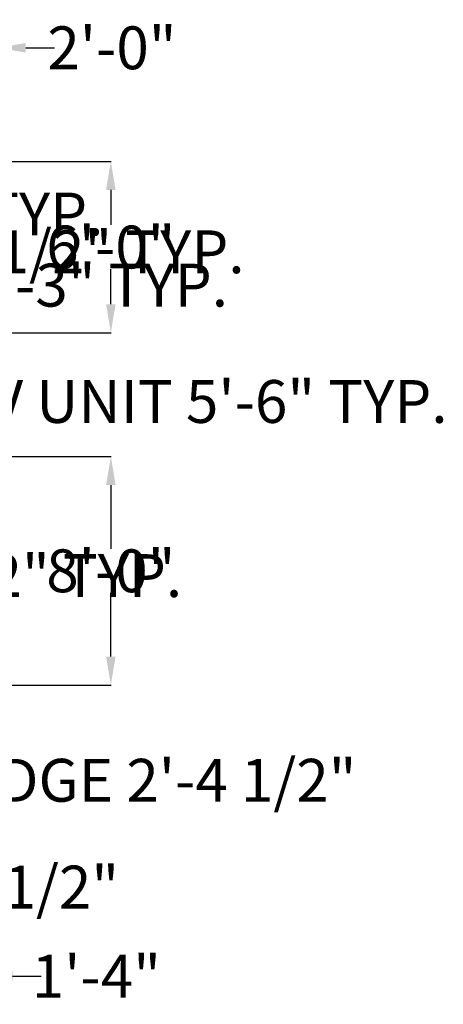
# Model space of a CAD drawing. Units: inches. Extents: x 2796 to 3603, y 978 to 1787.
# Tile 15 of 15: x 3425 to 3603, y 1374 to 1787. Entities that reach past the tile are written whole.
import ezdxf

# ---------------------------------------------------------------- set-up
doc = ezdxf.new("R2010")
doc.units = ezdxf.units.IN
doc.layers.add('A-ANNO-DIMS', color=7, linetype='Continuous', lineweight=18)
doc.styles.get("Standard").update_dxf_attribs({"font": 'arial.ttf'})
doc.dimstyles.get("Standard").update_dxf_attribs({"dimtxt": 18, "dimasz": 12, "dimexe": 0.18, "dimexo": 0.0625, "dimgap": 0.09, "dimtad": 0, "dimtih": 1, "dimtoh": 1, "dimdec": 0, "dimzin": 0, "dimdsep": 46, "dimlunit": 3, "dimtxsty": 'Standard', "dimcen": 0.09, "dimadec": 0, "dimazin": 0, "dimtfac": 1, "dimtdec": 0, "dimtofl": 0, "dimtmove": 0, "dimatfit": 3, "dimfxl": 1, "dimtolj": 1, "dimtzin": 0, "dimarcsym": 0})

# ---------------------------------------------------------------- blocks, each defined once
blk = doc.blocks.new('*D18')
at = {"layer": 'A-ANNO-DIMS', "color": 0, "lineweight": -2, "transparency": 16777216}
for p, q in [((3250.87, 1541.68), (3250.87, 1553.68)), ((3250.87, 1553.68), (3262.87, 1553.68)), ((3245.31, 1541.68), (3251.05, 1541.68)), ((3250.87, 1516.18), (3250.87, 1529.68)), ((3245.31, 1504.18), (3251.05, 1504.18))]:
    blk.add_line(p, q, dxfattribs=at)
at = {"layer": 'A-ANNO-DIMS', "color": 0, "transparency": 16777216}
for points in [[(3248.87, 1529.68), (3252.87, 1529.68), (3250.87, 1541.68)], [(3248.87, 1516.18), (3252.87, 1516.18), (3250.87, 1504.18)]]:
    blk.add_solid(points, dxfattribs=at)
at = {"layer": 'Defpoints', "color": 0, "transparency": 16777216}
for p in [(3245.25, 1541.68), (3250.87, 1541.68), (3245.25, 1504.18)]:
    blk.add_point(p, dxfattribs=at)
at = {"layer": 'A-ANNO-DIMS', "color": 0, "transparency": 16777216, "insert": (3379.56, 1553.68), "char_height": 18, "attachment_point": 5}
blk.add_mtext('\\A1;DOOR 3\'-1 1/2" TYP.', dxfattribs=at)
blk = doc.blocks.new('*D20')
at = {"layer": 'A-ANNO-DIMS', "color": 0, "lineweight": -2, "transparency": 16777216}
for p, q in [((3277.07, 1677.68), (3277.07, 1689.68)), ((3277.07, 1689.68), (3289.07, 1689.68)), ((3273.31, 1677.68), (3277.25, 1677.68)), ((3277.07, 1664.18), (3277.07, 1665.68)), ((3273.31, 1652.18), (3277.25, 1652.18))]:
    blk.add_line(p, q, dxfattribs=at)
at = {"layer": 'A-ANNO-DIMS', "color": 0, "transparency": 16777216}
for points in [[(3275.07, 1665.68), (3279.07, 1665.68), (3277.07, 1677.68)], [(3275.07, 1664.18), (3279.07, 1664.18), (3277.07, 1652.18)]]:
    blk.add_solid(points, dxfattribs=at)
at = {"layer": 'Defpoints', "color": 0, "transparency": 16777216}
for p in [(3273.25, 1677.68), (3277.07, 1677.68), (3273.25, 1652.18)]:
    blk.add_point(p, dxfattribs=at)
at = {"layer": 'A-ANNO-DIMS', "color": 0, "transparency": 16777216, "insert": (3405.76, 1689.68), "char_height": 18, "attachment_point": 5}
blk.add_mtext('\\A1;DOOR 2\'-1 1/2" TYP.', dxfattribs=at)
blk = doc.blocks.new('*D25')
at = {"layer": 'A-ANNO-DIMS', "color": 0, "lineweight": -2, "transparency": 16777216}
for p, q in [((3376.89, 1729.3), (3376.89, 1741.3)), ((3381.83, 1717.3), (3376.71, 1717.3)), ((3381.83, 1693.83), (3376.71, 1693.83)), ((3376.89, 1681.83), (3376.89, 1669.83))]:
    blk.add_line(p, q, dxfattribs=at)
at = {"layer": 'A-ANNO-DIMS', "color": 0, "transparency": 16777216}
for points in [[(3374.89, 1729.3), (3378.89, 1729.3), (3376.89, 1717.3)], [(3374.89, 1681.83), (3378.89, 1681.83), (3376.89, 1693.83)]]:
    blk.add_solid(points, dxfattribs=at)
at = {"layer": 'Defpoints', "color": 0, "transparency": 16777216}
for p in [(3381.89, 1717.3), (3376.89, 1693.83), (3381.89, 1693.83)]:
    blk.add_point(p, dxfattribs=at)
at = {"layer": 'A-ANNO-DIMS', "color": 0, "transparency": 16777216, "insert": (3376.89, 1705.57), "char_height": 18, "attachment_point": 5}
blk.add_mtext('\\A1;1\'-11 1/2" TYP.', dxfattribs=at)
blk = doc.blocks.new('*D28')
at = {"layer": 'A-ANNO-DIMS', "color": 0, "lineweight": -2, "transparency": 16777216}
for p, q in [((3315.48, 1636.61), (3315.48, 1626.63)), ((3381.25, 1636.61), (3381.25, 1626.63)), ((3327.48, 1626.81), (3369.25, 1626.81)), ((3381.25, 1626.81), (3393.25, 1626.81))]:
    blk.add_line(p, q, dxfattribs=at)
at = {"layer": 'A-ANNO-DIMS', "color": 0, "transparency": 16777216}
for points in [[(3327.48, 1628.81), (3327.48, 1624.81), (3315.48, 1626.81)], [(3369.25, 1628.81), (3369.25, 1624.81), (3381.25, 1626.81)]]:
    blk.add_solid(points, dxfattribs=at)
at = {"layer": 'Defpoints', "color": 0, "transparency": 16777216}
for p in [(3315.48, 1636.68), (3381.25, 1636.68), (3381.25, 1626.81)]:
    blk.add_point(p, dxfattribs=at)
at = {"layer": 'A-ANNO-DIMS', "color": 0, "transparency": 16777216, "insert": (3500.81, 1626.81), "char_height": 18, "attachment_point": 5}
blk.add_mtext('\\A1;TV UNIT 5\'-6" TYP.', dxfattribs=at)
blk = doc.blocks.new('*D29')
at = {"layer": 'A-ANNO-DIMS', "color": 0, "lineweight": -2, "transparency": 16777216}
for p, q in [((3391.11, 1663.68), (3391.11, 1675.68)), ((3391.11, 1675.68), (3403.11, 1675.68)), ((3381.31, 1651.68), (3391.29, 1651.68)), ((3381.31, 1636.68), (3391.29, 1636.68)), ((3391.11, 1624.68), (3391.11, 1612.68))]:
    blk.add_line(p, q, dxfattribs=at)
at = {"layer": 'A-ANNO-DIMS', "color": 0, "transparency": 16777216}
for points in [[(3389.11, 1663.68), (3393.11, 1663.68), (3391.11, 1651.68)], [(3389.11, 1624.68), (3393.11, 1624.68), (3391.11, 1636.68)]]:
    blk.add_solid(points, dxfattribs=at)
at = {"layer": 'Defpoints', "color": 0, "transparency": 16777216}
for p in [(3381.25, 1651.68), (3391.11, 1651.68), (3381.25, 1636.68)]:
    blk.add_point(p, dxfattribs=at)
at = {"layer": 'A-ANNO-DIMS', "color": 0, "transparency": 16777216, "insert": (3457.21, 1675.68), "char_height": 18, "attachment_point": 5}
blk.add_mtext('\\A1;1\'-3" TYP.', dxfattribs=at)
blk = doc.blocks.new('*D37')
at = {"layer": 'A-ANNO-DIMS', "color": 0, "lineweight": -2, "transparency": 16777216}
for p, q in [((3393.85, 1390.43), (3393.85, 1385.21)), ((3409.69, 1390.43), (3409.69, 1385.21)), ((3381.85, 1385.39), (3369.85, 1385.39)), ((3421.69, 1385.39), (3433.69, 1385.39))]:
    blk.add_line(p, q, dxfattribs=at)
at = {"layer": 'A-ANNO-DIMS', "color": 0, "transparency": 16777216}
for points in [[(3381.85, 1387.39), (3381.85, 1383.39), (3393.85, 1385.39)], [(3421.69, 1387.39), (3421.69, 1383.39), (3409.69, 1385.39)]]:
    blk.add_solid(points, dxfattribs=at)
at = {"layer": 'Defpoints', "color": 0, "transparency": 16777216}
for p in [(3393.85, 1390.49), (3409.69, 1390.49), (3409.69, 1385.39)]:
    blk.add_point(p, dxfattribs=at)
at = {"layer": 'A-ANNO-DIMS', "color": 0, "transparency": 16777216, "insert": (3456.86, 1385.39), "char_height": 18, "attachment_point": 5}
blk.add_mtext('\\A1;1\'-4"', dxfattribs=at)
blk = doc.blocks.new('*D38')
at = {"layer": 'A-ANNO-DIMS', "color": 0, "lineweight": -2, "transparency": 16777216}
for p, q in [((3365.25, 1455.68), (3365.25, 1467.68)), ((3365.25, 1467.68), (3377.25, 1467.68)), ((3361.02, 1455.68), (3365.43, 1455.68)), ((3365.25, 1439.11), (3365.25, 1443.68)), ((3361.02, 1427.11), (3365.43, 1427.11))]:
    blk.add_line(p, q, dxfattribs=at)
at = {"layer": 'A-ANNO-DIMS', "color": 0, "transparency": 16777216}
for points in [[(3363.25, 1443.68), (3367.25, 1443.68), (3365.25, 1455.68)], [(3363.25, 1439.11), (3367.25, 1439.11), (3365.25, 1427.11)]]:
    blk.add_solid(points, dxfattribs=at)
at = {"layer": 'Defpoints', "color": 0, "transparency": 16777216}
for p in [(3360.96, 1455.68), (3365.25, 1455.68), (3360.96, 1427.11)]:
    blk.add_point(p, dxfattribs=at)
at = {"layer": 'A-ANNO-DIMS', "color": 0, "transparency": 16777216, "insert": (3472.71, 1467.68), "char_height": 18, "attachment_point": 5}
blk.add_mtext('\\A1;FRIDGE 2\'-4 1/2"', dxfattribs=at)
blk = doc.blocks.new('*D39')
at = {"layer": 'A-ANNO-DIMS', "color": 0, "lineweight": -2, "transparency": 16777216}
for p, q in [((3334.3, 1427.04), (3334.3, 1422.64)), ((3360.96, 1427.04), (3360.96, 1422.64)), ((3346.3, 1422.82), (3348.96, 1422.82)), ((3360.96, 1422.82), (3372.96, 1422.82))]:
    blk.add_line(p, q, dxfattribs=at)
at = {"layer": 'A-ANNO-DIMS', "color": 0, "transparency": 16777216}
for points in [[(3346.3, 1424.82), (3346.3, 1420.82), (3334.3, 1422.82)], [(3348.96, 1424.82), (3348.96, 1420.82), (3360.96, 1422.82)]]:
    blk.add_solid(points, dxfattribs=at)
at = {"layer": 'Defpoints', "color": 0, "transparency": 16777216}
for p in [(3334.3, 1427.11), (3360.96, 1427.11), (3360.96, 1422.82)]:
    blk.add_point(p, dxfattribs=at)
at = {"layer": 'A-ANNO-DIMS', "color": 0, "transparency": 16777216, "insert": (3418.1, 1422.82), "char_height": 18, "attachment_point": 5}
blk.add_mtext('\\A1;2\'-2 1/2"', dxfattribs=at)
blk = doc.blocks.new('*D48')
at = {"layer": 'A-ANNO-DIMS', "color": 0, "lineweight": -2, "transparency": 16777216}
for p, q in [((3321.31, 1727.68), (3463.13, 1727.68)), ((3462.95, 1715.68), (3462.95, 1700.96)), ((3462.95, 1667.68), (3462.95, 1682.4)), ((3321.31, 1655.68), (3463.13, 1655.68))]:
    blk.add_line(p, q, dxfattribs=at)
at = {"layer": 'A-ANNO-DIMS', "color": 0, "transparency": 16777216}
for points in [[(3460.95, 1715.68), (3464.95, 1715.68), (3462.95, 1727.68)], [(3460.95, 1667.68), (3464.95, 1667.68), (3462.95, 1655.68)]]:
    blk.add_solid(points, dxfattribs=at)
at = {"layer": 'Defpoints', "color": 0, "transparency": 16777216}
for p in [(3321.25, 1727.68), (3462.95, 1727.68), (3321.25, 1655.68)]:
    blk.add_point(p, dxfattribs=at)
at = {"layer": 'A-ANNO-DIMS', "color": 0, "transparency": 16777216, "insert": (3462.95, 1691.68), "char_height": 18, "attachment_point": 5}
blk.add_mtext('\\A1;6\'-0"', dxfattribs=at)
blk = doc.blocks.new('*D49')
at = {"layer": 'A-ANNO-DIMS', "color": 0, "lineweight": -2, "transparency": 16777216}
for p, q in [((3415.31, 1603.68), (3463.13, 1603.68)), ((3462.95, 1591.68), (3462.95, 1564.96)), ((3462.95, 1519.68), (3462.95, 1546.4)), ((3415.31, 1507.68), (3463.13, 1507.68))]:
    blk.add_line(p, q, dxfattribs=at)
at = {"layer": 'A-ANNO-DIMS', "color": 0, "transparency": 16777216}
for points in [[(3460.95, 1591.68), (3464.95, 1591.68), (3462.95, 1603.68)], [(3460.95, 1519.68), (3464.95, 1519.68), (3462.95, 1507.68)]]:
    blk.add_solid(points, dxfattribs=at)
at = {"layer": 'Defpoints', "color": 0, "transparency": 16777216}
for p in [(3415.25, 1603.68), (3462.95, 1603.68), (3415.25, 1507.68)]:
    blk.add_point(p, dxfattribs=at)
at = {"layer": 'A-ANNO-DIMS', "color": 0, "transparency": 16777216, "insert": (3462.95, 1555.68), "char_height": 18, "attachment_point": 5}
blk.add_mtext('\\A1;8\'-0"', dxfattribs=at)
blk = doc.blocks.new('*D50')
at = {"layer": 'A-ANNO-DIMS', "color": 0, "lineweight": -2, "transparency": 16777216}
for p, q in [((3379.25, 1775.38), (3367.25, 1775.38)), ((3391.25, 1603.74), (3391.25, 1775.56)), ((3415.25, 1603.74), (3415.25, 1775.56)), ((3427.25, 1775.38), (3439.25, 1775.38))]:
    blk.add_line(p, q, dxfattribs=at)
at = {"layer": 'A-ANNO-DIMS', "color": 0, "transparency": 16777216}
for points in [[(3379.25, 1777.38), (3379.25, 1773.38), (3391.25, 1775.38)], [(3427.25, 1777.38), (3427.25, 1773.38), (3415.25, 1775.38)]]:
    blk.add_solid(points, dxfattribs=at)
at = {"layer": 'Defpoints', "color": 0, "transparency": 16777216}
for p in [(3415.25, 1775.38), (3391.25, 1603.68), (3415.25, 1603.68)]:
    blk.add_point(p, dxfattribs=at)
at = {"layer": 'A-ANNO-DIMS', "color": 0, "transparency": 16777216, "insert": (3463.41, 1775.38), "char_height": 18, "attachment_point": 5}
blk.add_mtext('\\A1;2\'-0"', dxfattribs=at)
blk = doc.blocks.new('*D54')
at = {"layer": 'A-ANNO-DIMS', "color": 0, "lineweight": -2, "transparency": 16777216}
for p, q in [((3379.25, 1775.38), (3367.25, 1775.38)), ((3391.25, 1431.74), (3391.25, 1775.56)), ((3415.25, 1455.74), (3415.25, 1775.56)), ((3427.25, 1775.38), (3439.25, 1775.38))]:
    blk.add_line(p, q, dxfattribs=at)
at = {"layer": 'A-ANNO-DIMS', "color": 0, "transparency": 16777216}
for points in [[(3379.25, 1777.38), (3379.25, 1773.38), (3391.25, 1775.38)], [(3427.25, 1777.38), (3427.25, 1773.38), (3415.25, 1775.38)]]:
    blk.add_solid(points, dxfattribs=at)
at = {"layer": 'Defpoints', "color": 0, "transparency": 16777216}
for p in [(3415.25, 1775.38), (3415.25, 1455.68), (3391.25, 1431.68)]:
    blk.add_point(p, dxfattribs=at)
at = {"layer": 'A-ANNO-DIMS', "color": 0, "transparency": 16777216, "insert": (3463.41, 1775.38), "char_height": 18, "attachment_point": 5}
blk.add_mtext('\\A1;2\'-0"', dxfattribs=at)

msp = doc.modelspace()

# ---------------------------------------------------------------- dimensions: what is measured, and where the dimension line sits
at = {"layer": 'A-ANNO-DIMS'}
for base, p1, p2, picture, middle in [((3415.25, 1775.38), (3391.25, 1603.68), (3415.25, 1603.68), '*D50', (3463.41, 1775.38)), ((3415.25, 1775.38), (3391.25, 1431.68), (3415.25, 1455.68), '*D54', (3463.41, 1775.38)), ((3360.96, 1422.82), (3334.3, 1427.11), (3360.96, 1427.11), '*D39', (3418.1, 1422.82)), ((3409.69, 1385.39), (3393.85, 1390.49), (3409.69, 1390.49), '*D37', (3456.86, 1385.39))]:
    dim = msp.add_linear_dim(base=base, p1=p1, p2=p2, dimstyle='Standard', override={"dimdec": 1, "dimlfac": 1, "dimrnd": 0, "dimzin": 1, "dimdsep": 46, "dimlunit": 4, "dimfrac": 2}, dxfattribs=at)
    dim.commit()
    dim.dimension.update_dxf_attribs({"geometry": picture, "text_midpoint": middle})
for base, p1, p2, angle, text, picture, middle in [((3277.07, 1677.68), (3273.25, 1652.18), (3273.25, 1677.68), 90, 'DOOR <> TYP.', '*D20', (3405.76, 1689.68)), ((3376.89, 1693.83), (3381.89, 1717.3), (3381.89, 1693.83), 270, '<> TYP.', '*D25', (3376.89, 1705.57)), ((3391.11, 1651.68), (3381.25, 1636.68), (3381.25, 1651.68), 90, '<> TYP.', '*D29', (3457.21, 1675.68)), ((3250.87, 1541.68), (3245.25, 1504.18), (3245.25, 1541.68), 90, 'DOOR <> TYP.', '*D18', (3379.56, 1553.68)), ((3365.25, 1455.68), (3360.96, 1427.11), (3360.96, 1455.68), 90, 'FRIDGE <>', '*D38', (3472.71, 1467.68))]:
    dim = msp.add_linear_dim(base=base, p1=p1, p2=p2, angle=angle, text=text, dimstyle='Standard', override={"dimdec": 1, "dimlfac": 1, "dimrnd": 0, "dimzin": 1, "dimdsep": 46, "dimlunit": 4, "dimfrac": 2}, dxfattribs=at)
    dim.commit()
    dim.dimension.update_dxf_attribs({"geometry": picture, "text_midpoint": middle})
for base, p1, p2, picture, middle in [((3462.95, 1727.68), (3321.25, 1655.68), (3321.25, 1727.68), '*D48', (3462.95, 1691.68)), ((3462.95, 1603.68), (3415.25, 1507.68), (3415.25, 1603.68), '*D49', (3462.95, 1555.68))]:
    dim = msp.add_linear_dim(base=base, p1=p1, p2=p2, angle=90, dimstyle='Standard', override={"dimdec": 1, "dimlfac": 1, "dimrnd": 0, "dimzin": 1, "dimdsep": 46, "dimlunit": 4, "dimfrac": 2}, dxfattribs=at)
    dim.commit()
    dim.dimension.update_dxf_attribs({"geometry": picture, "text_midpoint": middle})
dim = msp.add_linear_dim(base=(3381.25, 1626.81), p1=(3315.48, 1636.68), p2=(3381.25, 1636.68), text='TV UNIT <> TYP.', dimstyle='Standard', override={"dimdec": 1, "dimlfac": 1, "dimrnd": 0, "dimzin": 1, "dimdsep": 46, "dimlunit": 4, "dimfrac": 2}, dxfattribs=at)
dim.commit()
dim.dimension.update_dxf_attribs({"geometry": '*D28', "text_midpoint": (3500.81, 1626.81)})

doc.saveas('drawing.dxf')
